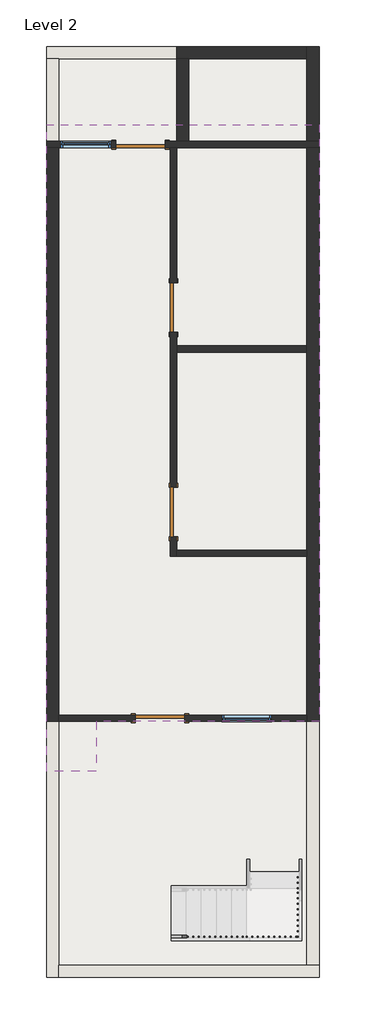
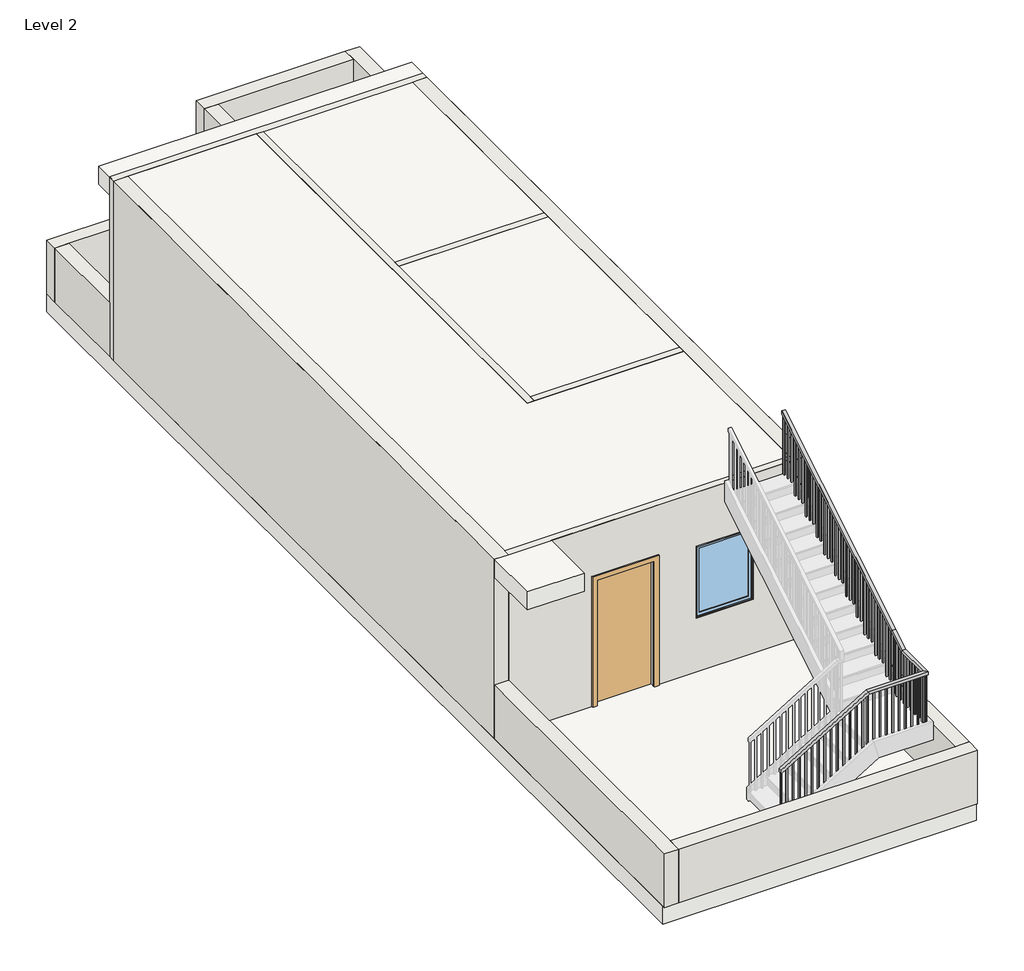
# One storey, part 1 of 2: 15 walls, 4 doors, 2 slabs, 2 windows, 1 railing.
"""IFC4 building model written with IfcOpenShell, lengths in millimetres."""

from ifc_helpers import new_model, si_unit, frame, origin, place, context, project, spatial, polyline, outline, extrude, faceted_brep, transform, mapped, element, save
from components import door_e5f9f3c4, window_41a96561

model = new_model("IFC4")

# Units and contexts
model_context = context("Model", 3, world=origin())
ifc_project = project(units=[si_unit("LENGTHUNIT", "METRE", prefix="MILLI")], contexts=[model_context])

# Site, building, storey
site = spatial("IfcSite", under=ifc_project)
building = spatial("IfcBuilding", under=site)
storey = spatial("IfcBuildingStorey", under=building, Name="Level 2", Elevation=3048.0)

# Doors
placement = place(None, origin())
door_shape = door_e5f9f3c4(model_context)
element("IfcDoor", 1, ObjectType="Single-Flush : 36\" x 84\"", at=placement, inside=storey, context=model_context, shape_type="MappedRepresentation", body=[
    mapped(door_shape, transform((-3555.9766939, -8657.0597562, 3048.0), x_axis=(1.0, 0.0, 0.0), y_axis=(0.0, 1.0, 0.0), z_axis=(0.0, 0.0, 1.0))),
])
element("IfcDoor", 2, ObjectType="Single-Flush : 36\" x 84\"", at=placement, inside=storey, context=model_context, shape_type="MappedRepresentation", body=[
    mapped(door_shape, transform((-3917.9266939, 1934.7402438, 3048.0), x_axis=(-1.0, 0.0, 0.0), y_axis=(0.0, -1.0, 0.0), z_axis=(0.0, 0.0, 1.0))),
])
element("IfcDoor", 3, ObjectType="Single-Flush : 36\" x 84\"", at=placement, inside=storey, context=model_context, shape_type="MappedRepresentation", body=[
    mapped(door_shape, transform((-3308.3266939, -1075.1597562, 3048.0), x_axis=(0.0, 1.0, 0.0), y_axis=(-1.0, 0.0, 0.0), z_axis=(0.0, 0.0, 1.0))),
])
element("IfcDoor", 4, ObjectType="Single-Flush : 36\" x 84\"", at=placement, inside=storey, context=model_context, shape_type="MappedRepresentation", body=[
    mapped(door_shape, transform((-3308.3266939, -4847.0597562, 3048.0), x_axis=(0.0, 1.0, 0.0), y_axis=(-1.0, 0.0, 0.0), z_axis=(0.0, 0.0, 1.0))),
])

# Railing
element("IfcRailing", 5, ObjectType="Handrail - Rectangular", at=placement, inside=storey, context=model_context, shape_type="SolidModel", body=[
    faceted_brep([(-3351.0563134, -12658.659218, 4131.7333333), (-3351.0563134, -12658.659218, 4072.3318731), (-3351.0563134, -12709.459218, 4072.3318731), (-3351.0563134, -12709.459218, 4131.7333333), (-1954.0563134, -12658.659218, 4978.4), (-1939.863904, -12658.659218, 4927.6), (-1939.863904, -12709.459218, 4927.6), (-1954.0563134, -12709.459218, 4978.4), (-1039.6563134, -12658.659218, 4978.4), (-1039.6563134, -12658.659218, 4927.6), (-988.8563134, -12709.459218, 4927.6), (-988.8563134, -12709.459218, 4978.4), (-1039.6563134, -12074.459218, 4978.4), (-1039.6563134, -12060.2668086, 4927.6), (-988.8563134, -12060.2668086, 4927.6), (-988.8563134, -12074.459218, 4978.4), (-1039.6563134, -11795.059218, 5147.7333333), (-1039.6563134, -11768.7294908, 5104.2892835), (-988.8563134, -11768.7294908, 5104.2892835), (-988.8563134, -11795.059218, 5147.7333333), (-1039.6563134, -8721.659218, 7010.4), (-988.8563134, -8721.659218, 7010.4), (-988.8563134, -8721.659218, 6950.9985397), (-1039.6563134, -8721.659218, 6950.9985397)], [[[0, 1, 2, 3]], [[1, 0, 4, 5]], [[2, 1, 5, 6]], [[3, 2, 6, 7]], [[0, 3, 7, 4]], [[5, 4, 8, 9]], [[6, 5, 9, 10]], [[7, 6, 10, 11]], [[4, 7, 11, 8]], [[9, 8, 12, 13]], [[10, 9, 13, 14]], [[11, 10, 14, 15]], [[8, 11, 15, 12]], [[13, 12, 16, 17]], [[14, 13, 17, 18]], [[15, 14, 18, 19]], [[12, 15, 19, 16]], [[20, 21, 22, 23]], [[17, 16, 20, 23]], [[18, 17, 23, 22]], [[19, 18, 22, 21]], [[16, 19, 21, 20]]]),
    extrude(outline(polyline([(-8756.584218, 6929.8318731), (-8737.534218, 6941.3773276), (-8737.534218, 5926.6666667), (-8756.584218, 5926.6666667), (-8756.584218, 6929.8318731)])), frame((-1023.7813134, 0.0, 0.0), z_axis=(1.0, 0.0, 0.0), x_axis=(0.0, 1.0, 0.0)), (0.0, 0.0, 1.0), 19.05),
    extrude(outline(polyline([(-8858.184218, 6868.2561155), (-8839.134218, 6879.80157), (-8839.134218, 5926.6666667), (-8858.184218, 5926.6666667), (-8858.184218, 6868.2561155)])), frame((-1023.7813134, 0.0, 0.0), z_axis=(1.0, 0.0, 0.0), x_axis=(0.0, 1.0, 0.0)), (0.0, 0.0, 1.0), 19.05),
    extrude(outline(polyline([(-8959.784218, 6806.6803579), (-8940.734218, 6818.2258125), (-8940.734218, 5926.6666667), (-8959.784218, 5926.6666667), (-8959.784218, 6806.6803579)])), frame((-1023.7813134, 0.0, 0.0), z_axis=(1.0, 0.0, 0.0), x_axis=(0.0, 1.0, 0.0)), (0.0, 0.0, 1.0), 19.05),
    extrude(outline(polyline([(-9061.384218, 6745.1046004), (-9042.334218, 6756.6500549), (-9042.334218, 5757.3333333), (-9061.384218, 5757.3333333), (-9061.384218, 6745.1046004)])), frame((-1023.7813134, 0.0, 0.0), z_axis=(1.0, 0.0, 0.0), x_axis=(0.0, 1.0, 0.0)), (0.0, 0.0, 1.0), 19.05),
    extrude(outline(polyline([(-9162.984218, 6683.5288428), (-9143.934218, 6695.0742973), (-9143.934218, 5757.3333333), (-9162.984218, 5757.3333333), (-9162.984218, 6683.5288428)])), frame((-1023.7813134, 0.0, 0.0), z_axis=(1.0, 0.0, 0.0), x_axis=(0.0, 1.0, 0.0)), (0.0, 0.0, 1.0), 19.05),
    extrude(outline(polyline([(-9264.584218, 6621.9530852), (-9245.534218, 6633.4985397), (-9245.534218, 5757.3333333), (-9264.584218, 5757.3333333), (-9264.584218, 6621.9530852)])), frame((-1023.7813134, 0.0, 0.0), z_axis=(1.0, 0.0, 0.0), x_axis=(0.0, 1.0, 0.0)), (0.0, 0.0, 1.0), 19.05),
    extrude(outline(polyline([(-9366.184218, 6560.3773276), (-9347.134218, 6571.9227822), (-9347.134218, 5588.0), (-9366.184218, 5588.0), (-9366.184218, 6560.3773276)])), frame((-1023.7813134, 0.0, 0.0), z_axis=(1.0, 0.0, 0.0), x_axis=(0.0, 1.0, 0.0)), (0.0, 0.0, 1.0), 19.05),
    extrude(outline(polyline([(-9467.784218, 6498.80157), (-9448.734218, 6510.3470246), (-9448.734218, 5588.0), (-9467.784218, 5588.0), (-9467.784218, 6498.80157)])), frame((-1023.7813134, 0.0, 0.0), z_axis=(1.0, 0.0, 0.0), x_axis=(0.0, 1.0, 0.0)), (0.0, 0.0, 1.0), 19.05),
    extrude(outline(polyline([(-9569.384218, 6437.2258125), (-9550.334218, 6448.771267), (-9550.334218, 5588.0), (-9569.384218, 5588.0), (-9569.384218, 6437.2258125)])), frame((-1023.7813134, 0.0, 0.0), z_axis=(1.0, 0.0, 0.0), x_axis=(0.0, 1.0, 0.0)), (0.0, 0.0, 1.0), 19.05),
    extrude(outline(polyline([(-9670.984218, 6375.6500549), (-9651.934218, 6387.1955094), (-9651.934218, 5418.6666667), (-9670.984218, 5418.6666667), (-9670.984218, 6375.6500549)])), frame((-1023.7813134, 0.0, 0.0), z_axis=(1.0, 0.0, 0.0), x_axis=(0.0, 1.0, 0.0)), (0.0, 0.0, 1.0), 19.05),
    extrude(outline(polyline([(-9772.584218, 6314.0742973), (-9753.534218, 6325.6197519), (-9753.534218, 5418.6666667), (-9772.584218, 5418.6666667), (-9772.584218, 6314.0742973)])), frame((-1023.7813134, 0.0, 0.0), z_axis=(1.0, 0.0, 0.0), x_axis=(0.0, 1.0, 0.0)), (0.0, 0.0, 1.0), 19.05),
    extrude(outline(polyline([(-9874.184218, 6252.4985397), (-9855.134218, 6264.0439943), (-9855.134218, 5249.3333333), (-9874.184218, 5249.3333333), (-9874.184218, 6252.4985397)])), frame((-1023.7813134, 0.0, 0.0), z_axis=(1.0, 0.0, 0.0), x_axis=(0.0, 1.0, 0.0)), (0.0, 0.0, 1.0), 19.05),
    extrude(outline(polyline([(-9975.784218, 6190.9227822), (-9956.734218, 6202.4682367), (-9956.734218, 5249.3333333), (-9975.784218, 5249.3333333), (-9975.784218, 6190.9227822)])), frame((-1023.7813134, 0.0, 0.0), z_axis=(1.0, 0.0, 0.0), x_axis=(0.0, 1.0, 0.0)), (0.0, 0.0, 1.0), 19.05),
    extrude(outline(polyline([(-10077.384218, 6129.3470246), (-10058.334218, 6140.8924791), (-10058.334218, 5249.3333333), (-10077.384218, 5249.3333333), (-10077.384218, 6129.3470246)])), frame((-1023.7813134, 0.0, 0.0), z_axis=(1.0, 0.0, 0.0), x_axis=(0.0, 1.0, 0.0)), (0.0, 0.0, 1.0), 19.05),
    extrude(outline(polyline([(-10178.984218, 6067.771267), (-10159.934218, 6079.3167216), (-10159.934218, 5080.0), (-10178.984218, 5080.0), (-10178.984218, 6067.771267)])), frame((-1023.7813134, 0.0, 0.0), z_axis=(1.0, 0.0, 0.0), x_axis=(0.0, 1.0, 0.0)), (0.0, 0.0, 1.0), 19.05),
    extrude(outline(polyline([(-10280.584218, 6006.1955094), (-10261.534218, 6017.740964), (-10261.534218, 5080.0), (-10280.584218, 5080.0), (-10280.584218, 6006.1955094)])), frame((-1023.7813134, 0.0, 0.0), z_axis=(1.0, 0.0, 0.0), x_axis=(0.0, 1.0, 0.0)), (0.0, 0.0, 1.0), 19.05),
    extrude(outline(polyline([(-10382.184218, 5944.6197519), (-10363.134218, 5956.1652064), (-10363.134218, 5080.0), (-10382.184218, 5080.0), (-10382.184218, 5944.6197519)])), frame((-1023.7813134, 0.0, 0.0), z_axis=(1.0, 0.0, 0.0), x_axis=(0.0, 1.0, 0.0)), (0.0, 0.0, 1.0), 19.05),
    extrude(outline(polyline([(-10483.784218, 5883.0439943), (-10464.734218, 5894.5894488), (-10464.734218, 4910.6666667), (-10483.784218, 4910.6666667), (-10483.784218, 5883.0439943)])), frame((-1023.7813134, 0.0, 0.0), z_axis=(1.0, 0.0, 0.0), x_axis=(0.0, 1.0, 0.0)), (0.0, 0.0, 1.0), 19.05),
    extrude(outline(polyline([(-10585.384218, 5821.4682367), (-10566.334218, 5833.0136913), (-10566.334218, 4910.6666667), (-10585.384218, 4910.6666667), (-10585.384218, 5821.4682367)])), frame((-1023.7813134, 0.0, 0.0), z_axis=(1.0, 0.0, 0.0), x_axis=(0.0, 1.0, 0.0)), (0.0, 0.0, 1.0), 19.05),
    extrude(outline(polyline([(-10686.984218, 5759.8924791), (-10667.934218, 5771.4379337), (-10667.934218, 4910.6666667), (-10686.984218, 4910.6666667), (-10686.984218, 5759.8924791)])), frame((-1023.7813134, 0.0, 0.0), z_axis=(1.0, 0.0, 0.0), x_axis=(0.0, 1.0, 0.0)), (0.0, 0.0, 1.0), 19.05),
    extrude(outline(polyline([(-10788.584218, 5698.3167216), (-10769.534218, 5709.8621761), (-10769.534218, 4741.3333333), (-10788.584218, 4741.3333333), (-10788.584218, 5698.3167216)])), frame((-1023.7813134, 0.0, 0.0), z_axis=(1.0, 0.0, 0.0), x_axis=(0.0, 1.0, 0.0)), (0.0, 0.0, 1.0), 19.05),
    extrude(outline(polyline([(-10890.184218, 5636.740964), (-10871.134218, 5648.2864185), (-10871.134218, 4741.3333333), (-10890.184218, 4741.3333333), (-10890.184218, 5636.740964)])), frame((-1023.7813134, 0.0, 0.0), z_axis=(1.0, 0.0, 0.0), x_axis=(0.0, 1.0, 0.0)), (0.0, 0.0, 1.0), 19.05),
    extrude(outline(polyline([(-10991.784218, 5575.1652064), (-10972.734218, 5586.710661), (-10972.734218, 4572.0), (-10991.784218, 4572.0), (-10991.784218, 5575.1652064)])), frame((-1023.7813134, 0.0, 0.0), z_axis=(1.0, 0.0, 0.0), x_axis=(0.0, 1.0, 0.0)), (0.0, 0.0, 1.0), 19.05),
    extrude(outline(polyline([(-11093.384218, 5513.5894488), (-11074.334218, 5525.1349034), (-11074.334218, 4572.0), (-11093.384218, 4572.0), (-11093.384218, 5513.5894488)])), frame((-1023.7813134, 0.0, 0.0), z_axis=(1.0, 0.0, 0.0), x_axis=(0.0, 1.0, 0.0)), (0.0, 0.0, 1.0), 19.05),
    extrude(outline(polyline([(-11194.984218, 5452.0136913), (-11175.934218, 5463.5591458), (-11175.934218, 4572.0), (-11194.984218, 4572.0), (-11194.984218, 5452.0136913)])), frame((-1023.7813134, 0.0, 0.0), z_axis=(1.0, 0.0, 0.0), x_axis=(0.0, 1.0, 0.0)), (0.0, 0.0, 1.0), 19.05),
    extrude(outline(polyline([(-11296.584218, 5390.4379337), (-11277.534218, 5401.9833882), (-11277.534218, 4402.6666667), (-11296.584218, 4402.6666667), (-11296.584218, 5390.4379337)])), frame((-1023.7813134, 0.0, 0.0), z_axis=(1.0, 0.0, 0.0), x_axis=(0.0, 1.0, 0.0)), (0.0, 0.0, 1.0), 19.05),
    extrude(outline(polyline([(-11398.184218, 5328.8621761), (-11379.134218, 5340.4076307), (-11379.134218, 4402.6666667), (-11398.184218, 4402.6666667), (-11398.184218, 5328.8621761)])), frame((-1023.7813134, 0.0, 0.0), z_axis=(1.0, 0.0, 0.0), x_axis=(0.0, 1.0, 0.0)), (0.0, 0.0, 1.0), 19.05),
    extrude(outline(polyline([(-11499.784218, 5267.2864185), (-11480.734218, 5278.8318731), (-11480.734218, 4402.6666667), (-11499.784218, 4402.6666667), (-11499.784218, 5267.2864185)])), frame((-1023.7813134, 0.0, 0.0), z_axis=(1.0, 0.0, 0.0), x_axis=(0.0, 1.0, 0.0)), (0.0, 0.0, 1.0), 19.05),
    extrude(outline(polyline([(-11601.384218, 5205.710661), (-11582.334218, 5217.2561155), (-11582.334218, 4233.3333333), (-11601.384218, 4233.3333333), (-11601.384218, 5205.710661)])), frame((-1023.7813134, 0.0, 0.0), z_axis=(1.0, 0.0, 0.0), x_axis=(0.0, 1.0, 0.0)), (0.0, 0.0, 1.0), 19.05),
    extrude(outline(polyline([(-11702.984218, 5144.1349034), (-11683.934218, 5155.6803579), (-11683.934218, 4233.3333333), (-11702.984218, 4233.3333333), (-11702.984218, 5144.1349034)])), frame((-1023.7813134, 0.0, 0.0), z_axis=(1.0, 0.0, 0.0), x_axis=(0.0, 1.0, 0.0)), (0.0, 0.0, 1.0), 19.05),
    extrude(outline(polyline([(-11880.784218, 5036.3773276), (-11861.734218, 5047.9227822), (-11861.734218, 4064.0), (-11880.784218, 4064.0), (-11880.784218, 5036.3773276)])), frame((-1023.7813134, 0.0, 0.0), z_axis=(1.0, 0.0, 0.0), x_axis=(0.0, 1.0, 0.0)), (0.0, 0.0, 1.0), 19.05),
    extrude(outline(polyline([(-11982.384218, 4974.80157), (-11963.334218, 4986.3470246), (-11963.334218, 4064.0), (-11982.384218, 4064.0), (-11982.384218, 4974.80157)])), frame((-1023.7813134, 0.0, 0.0), z_axis=(1.0, 0.0, 0.0), x_axis=(0.0, 1.0, 0.0)), (0.0, 0.0, 1.0), 19.05),
    extrude(outline(polyline([(-1004.7313134, -12083.984218), (-1023.7813134, -12083.984218), (-1023.7813134, -12064.934218), (-1004.7313134, -12064.934218), (-1004.7313134, -12083.984218)])), frame((0.0, 0.0, 4064.0), z_axis=(0.0, 0.0, 1.0), x_axis=(1.0, 0.0, 0.0)), (0.0, 0.0, 1.0), 863.6),
    extrude(outline(polyline([(-1004.7313134, -12185.584218), (-1023.7813134, -12185.584218), (-1023.7813134, -12166.534218), (-1004.7313134, -12166.534218), (-1004.7313134, -12185.584218)])), frame((0.0, 0.0, 4064.0), z_axis=(0.0, 0.0, 1.0), x_axis=(1.0, 0.0, 0.0)), (0.0, 0.0, 1.0), 863.6),
    extrude(outline(polyline([(-1004.7313134, -12287.184218), (-1023.7813134, -12287.184218), (-1023.7813134, -12268.134218), (-1004.7313134, -12268.134218), (-1004.7313134, -12287.184218)])), frame((0.0, 0.0, 4064.0), z_axis=(0.0, 0.0, 1.0), x_axis=(1.0, 0.0, 0.0)), (0.0, 0.0, 1.0), 863.6),
    extrude(outline(polyline([(-1004.7313134, -12388.784218), (-1023.7813134, -12388.784218), (-1023.7813134, -12369.734218), (-1004.7313134, -12369.734218), (-1004.7313134, -12388.784218)])), frame((0.0, 0.0, 4064.0), z_axis=(0.0, 0.0, 1.0), x_axis=(1.0, 0.0, 0.0)), (0.0, 0.0, 1.0), 863.6),
    extrude(outline(polyline([(-1004.7313134, -12490.384218), (-1023.7813134, -12490.384218), (-1023.7813134, -12471.334218), (-1004.7313134, -12471.334218), (-1004.7313134, -12490.384218)])), frame((0.0, 0.0, 4064.0), z_axis=(0.0, 0.0, 1.0), x_axis=(1.0, 0.0, 0.0)), (0.0, 0.0, 1.0), 863.6),
    extrude(outline(polyline([(-1004.7313134, -12591.984218), (-1023.7813134, -12591.984218), (-1023.7813134, -12572.934218), (-1004.7313134, -12572.934218), (-1004.7313134, -12591.984218)])), frame((0.0, 0.0, 4064.0), z_axis=(0.0, 0.0, 1.0), x_axis=(1.0, 0.0, 0.0)), (0.0, 0.0, 1.0), 863.6),
    extrude(outline(polyline([(-1049.1813134, -12693.584218), (-1049.1813134, -12674.534218), (-1030.1313134, -12674.534218), (-1030.1313134, -12693.584218), (-1049.1813134, -12693.584218)])), frame((0.0, 0.0, 4064.0), z_axis=(0.0, 0.0, 1.0), x_axis=(1.0, 0.0, 0.0)), (0.0, 0.0, 1.0), 863.6),
    extrude(outline(polyline([(-1150.7813134, -12693.584218), (-1150.7813134, -12674.534218), (-1131.7313134, -12674.534218), (-1131.7313134, -12693.584218), (-1150.7813134, -12693.584218)])), frame((0.0, 0.0, 4064.0), z_axis=(0.0, 0.0, 1.0), x_axis=(1.0, 0.0, 0.0)), (0.0, 0.0, 1.0), 863.6),
    extrude(outline(polyline([(-1252.3813134, -12693.584218), (-1252.3813134, -12674.534218), (-1233.3313134, -12674.534218), (-1233.3313134, -12693.584218), (-1252.3813134, -12693.584218)])), frame((0.0, 0.0, 4064.0), z_axis=(0.0, 0.0, 1.0), x_axis=(1.0, 0.0, 0.0)), (0.0, 0.0, 1.0), 863.6),
    extrude(outline(polyline([(-1353.9813134, -12693.584218), (-1353.9813134, -12674.534218), (-1334.9313134, -12674.534218), (-1334.9313134, -12693.584218), (-1353.9813134, -12693.584218)])), frame((0.0, 0.0, 4064.0), z_axis=(0.0, 0.0, 1.0), x_axis=(1.0, 0.0, 0.0)), (0.0, 0.0, 1.0), 863.6),
    extrude(outline(polyline([(-1455.5813134, -12693.584218), (-1455.5813134, -12674.534218), (-1436.5313134, -12674.534218), (-1436.5313134, -12693.584218), (-1455.5813134, -12693.584218)])), frame((0.0, 0.0, 4064.0), z_axis=(0.0, 0.0, 1.0), x_axis=(1.0, 0.0, 0.0)), (0.0, 0.0, 1.0), 863.6),
    extrude(outline(polyline([(-1557.1813134, -12693.584218), (-1557.1813134, -12674.534218), (-1538.1313134, -12674.534218), (-1538.1313134, -12693.584218), (-1557.1813134, -12693.584218)])), frame((0.0, 0.0, 4064.0), z_axis=(0.0, 0.0, 1.0), x_axis=(1.0, 0.0, 0.0)), (0.0, 0.0, 1.0), 863.6),
    extrude(outline(polyline([(-1658.7813134, -12693.584218), (-1658.7813134, -12674.534218), (-1639.7313134, -12674.534218), (-1639.7313134, -12693.584218), (-1658.7813134, -12693.584218)])), frame((0.0, 0.0, 4064.0), z_axis=(0.0, 0.0, 1.0), x_axis=(1.0, 0.0, 0.0)), (0.0, 0.0, 1.0), 863.6),
    extrude(outline(polyline([(-1760.3813134, -12693.584218), (-1760.3813134, -12674.534218), (-1741.3313134, -12674.534218), (-1741.3313134, -12693.584218), (-1760.3813134, -12693.584218)])), frame((0.0, 0.0, 4064.0), z_axis=(0.0, 0.0, 1.0), x_axis=(1.0, 0.0, 0.0)), (0.0, 0.0, 1.0), 863.6),
    extrude(outline(polyline([(-1861.9813134, -12693.584218), (-1861.9813134, -12674.534218), (-1842.9313134, -12674.534218), (-1842.9313134, -12693.584218), (-1861.9813134, -12693.584218)])), frame((0.0, 0.0, 4064.0), z_axis=(0.0, 0.0, 1.0), x_axis=(1.0, 0.0, 0.0)), (0.0, 0.0, 1.0), 863.6),
    extrude(outline(polyline([(4878.5894488, -2020.7313134), (4867.0439943, -2039.7813134), (3894.6666667, -2039.7813134), (3894.6666667, -2020.7313134), (4878.5894488, -2020.7313134)])), frame((0.0, -12693.584218, 0.0), z_axis=(0.0, 1.0, 0.0), x_axis=(0.0, 0.0, 1.0)), (0.0, 0.0, 1.0), 19.05),
    extrude(outline(polyline([(4817.0136913, -2122.3313134), (4805.4682367, -2141.3813134), (3894.6666667, -2141.3813134), (3894.6666667, -2122.3313134), (4817.0136913, -2122.3313134)])), frame((0.0, -12693.584218, 0.0), z_axis=(0.0, 1.0, 0.0), x_axis=(0.0, 0.0, 1.0)), (0.0, 0.0, 1.0), 19.05),
    extrude(outline(polyline([(4755.4379337, -2223.9313134), (4743.8924791, -2242.9813134), (3894.6666667, -2242.9813134), (3894.6666667, -2223.9313134), (4755.4379337, -2223.9313134)])), frame((0.0, -12693.584218, 0.0), z_axis=(0.0, 1.0, 0.0), x_axis=(0.0, 0.0, 1.0)), (0.0, 0.0, 1.0), 19.05),
    extrude(outline(polyline([(4693.8621761, -2325.5313134), (4682.3167216, -2344.5813134), (3725.3333333, -2344.5813134), (3725.3333333, -2325.5313134), (4693.8621761, -2325.5313134)])), frame((0.0, -12693.584218, 0.0), z_axis=(0.0, 1.0, 0.0), x_axis=(0.0, 0.0, 1.0)), (0.0, 0.0, 1.0), 19.05),
    extrude(outline(polyline([(4632.2864185, -2427.1313134), (4620.740964, -2446.1813134), (3725.3333333, -2446.1813134), (3725.3333333, -2427.1313134), (4632.2864185, -2427.1313134)])), frame((0.0, -12693.584218, 0.0), z_axis=(0.0, 1.0, 0.0), x_axis=(0.0, 0.0, 1.0)), (0.0, 0.0, 1.0), 19.05),
    extrude(outline(polyline([(4570.710661, -2528.7313134), (4559.1652064, -2547.7813134), (3556.0, -2547.7813134), (3556.0, -2528.7313134), (4570.710661, -2528.7313134)])), frame((0.0, -12693.584218, 0.0), z_axis=(0.0, 1.0, 0.0), x_axis=(0.0, 0.0, 1.0)), (0.0, 0.0, 1.0), 19.05),
    extrude(outline(polyline([(4509.1349034, -2630.3313134), (4497.5894488, -2649.3813134), (3556.0, -2649.3813134), (3556.0, -2630.3313134), (4509.1349034, -2630.3313134)])), frame((0.0, -12693.584218, 0.0), z_axis=(0.0, 1.0, 0.0), x_axis=(0.0, 0.0, 1.0)), (0.0, 0.0, 1.0), 19.05),
    extrude(outline(polyline([(4447.5591458, -2731.9313134), (4436.0136913, -2750.9813134), (3556.0, -2750.9813134), (3556.0, -2731.9313134), (4447.5591458, -2731.9313134)])), frame((0.0, -12693.584218, 0.0), z_axis=(0.0, 1.0, 0.0), x_axis=(0.0, 0.0, 1.0)), (0.0, 0.0, 1.0), 19.05),
    extrude(outline(polyline([(4385.9833882, -2833.5313134), (4374.4379337, -2852.5813134), (3386.6666667, -2852.5813134), (3386.6666667, -2833.5313134), (4385.9833882, -2833.5313134)])), frame((0.0, -12693.584218, 0.0), z_axis=(0.0, 1.0, 0.0), x_axis=(0.0, 0.0, 1.0)), (0.0, 0.0, 1.0), 19.05),
    extrude(outline(polyline([(4324.4076307, -2935.1313134), (4312.8621761, -2954.1813134), (3386.6666667, -2954.1813134), (3386.6666667, -2935.1313134), (4324.4076307, -2935.1313134)])), frame((0.0, -12693.584218, 0.0), z_axis=(0.0, 1.0, 0.0), x_axis=(0.0, 0.0, 1.0)), (0.0, 0.0, 1.0), 19.05),
    extrude(outline(polyline([(4262.8318731, -3036.7313134), (4251.2864185, -3055.7813134), (3386.6666667, -3055.7813134), (3386.6666667, -3036.7313134), (4262.8318731, -3036.7313134)])), frame((0.0, -12693.584218, 0.0), z_axis=(0.0, 1.0, 0.0), x_axis=(0.0, 0.0, 1.0)), (0.0, 0.0, 1.0), 19.05),
    extrude(outline(polyline([(4201.2561155, -3138.3313134), (4189.710661, -3157.3813134), (3217.3333333, -3157.3813134), (3217.3333333, -3138.3313134), (4201.2561155, -3138.3313134)])), frame((0.0, -12693.584218, 0.0), z_axis=(0.0, 1.0, 0.0), x_axis=(0.0, 0.0, 1.0)), (0.0, 0.0, 1.0), 19.05),
    extrude(outline(polyline([(4139.6803579, -3239.9313134), (4128.1349034, -3258.9813134), (3217.3333333, -3258.9813134), (3217.3333333, -3239.9313134), (4139.6803579, -3239.9313134)])), frame((0.0, -12693.584218, 0.0), z_axis=(0.0, 1.0, 0.0), x_axis=(0.0, 0.0, 1.0)), (0.0, 0.0, 1.0), 19.05),
    extrude(outline(polyline([(-11804.584218, 5082.5591458), (-11785.534218, 5094.1046004), (-11785.534218, 4064.0), (-11804.584218, 4064.0), (-11804.584218, 5082.5591458)])), frame((-1023.7813134, 0.0, 0.0), z_axis=(1.0, 0.0, 0.0), x_axis=(0.0, 1.0, 0.0)), (0.0, 0.0, 1.0), 19.05),
    extrude(outline(polyline([(-1023.7813134, -12693.584218), (-1023.7813134, -12674.534218), (-1004.7313134, -12674.534218), (-1004.7313134, -12693.584218), (-1023.7813134, -12693.584218)])), frame((0.0, 0.0, 4064.0), z_axis=(0.0, 0.0, 1.0), x_axis=(1.0, 0.0, 0.0)), (0.0, 0.0, 1.0), 863.6),
    extrude(outline(polyline([(4924.771267, -1944.5313134), (4913.2258125, -1963.5813134), (4064.0, -1963.5813134), (4064.0, -1944.5313134), (4924.771267, -1944.5313134)])), frame((0.0, -12693.584218, 0.0), z_axis=(0.0, 1.0, 0.0), x_axis=(0.0, 0.0, 1.0)), (0.0, 0.0, 1.0), 19.05),
    extrude(outline(polyline([(-8740.709218, 6939.4530852), (-8721.659218, 6950.9985397), (-8721.659218, 5926.6666667), (-8740.709218, 5926.6666667), (-8740.709218, 6939.4530852)])), frame((-1023.7813134, 0.0, 0.0), z_axis=(1.0, 0.0, 0.0), x_axis=(0.0, 1.0, 0.0)), (0.0, 0.0, 1.0), 19.05),
    extrude(outline(polyline([(4083.8773276, -3332.0063134), (4072.3318731, -3351.0563134), (3217.3333333, -3351.0563134), (3217.3333333, -3332.0063134), (4083.8773276, -3332.0063134)])), frame((0.0, -12693.584218, 0.0), z_axis=(0.0, 1.0, 0.0), x_axis=(0.0, 0.0, 1.0)), (0.0, 0.0, 1.0), 19.05),
])

# Slabs
element("IfcSlab", 6, ObjectType="slab 6\"", at=placement, inside=storey, context=model_context, shape_type="SweptSolid", body=[
    extrude(outline(polyline([(-622.2766939, 3744.4902438), (-622.2766939, -13400.5097562), (-5651.4766939, -13400.5097562), (-5651.4766939, 3744.4902438), (-622.2766939, 3744.4902438)])), frame((0.0, 0.0, 2743.2), z_axis=(0.0, 0.0, 1.0), x_axis=(1.0, 0.0, 0.0)), (0.0, 0.0, 1.0), 304.8),
])
element("IfcSlab", 7, ObjectType="slab 6\"", at=placement, inside=storey, context=model_context, shape_type="SweptSolid", body=[
    extrude(outline(polyline([(-622.2766939, 2296.6902438), (-622.2766939, -8714.2097562), (-4737.0766939, -8714.2097562), (-4737.0766939, -9628.6097562), (-5651.4766939, -9628.6097562), (-5651.4766939, -8714.2097562), (-5651.4766939, 2296.6902438), (-622.2766939, 2296.6902438)])), frame((0.0, 0.0, 5791.2), z_axis=(0.0, 0.0, 1.0), x_axis=(1.0, 0.0, 0.0)), (0.0, 0.0, 1.0), 304.8),
])

# Walls
element("IfcWall", 8, ObjectType="wall 4.5\"", at=placement, inside=storey, context=model_context, shape_type="Brep", body=[
    faceted_brep([(-5651.4766939, 1877.5902438, 3048.0), (-5422.8766939, 1877.5902438, 3048.0), (-4375.1266939, 1877.5902438, 3048.0), (-4375.1266939, 1877.5902438, 5181.6), (-3460.7266939, 1877.5902438, 5181.6), (-3460.7266939, 1877.5902438, 3048.0), (-3365.4766939, 1877.5902438, 3048.0), (-3251.1766939, 1877.5902438, 3048.0), (-850.8766939, 1877.5902438, 3048.0), (-622.2766939, 1877.5902438, 3048.0), (-622.2766939, 1877.5902438, 6096.0), (-850.8766939, 1877.5902438, 6096.0), (-3251.1766939, 1877.5902438, 6096.0), (-3365.4766939, 1877.5902438, 6096.0), (-5422.8766939, 1877.5902438, 6096.0), (-5651.4766939, 1877.5902438, 6096.0), (-4470.3766939, 1877.5902438, 5181.6), (-4470.3766939, 1877.5902438, 3962.4), (-5384.7766939, 1877.5902438, 3962.4), (-5384.7766939, 1877.5902438, 5181.6), (-4375.1266939, 1991.8902438, 5181.6), (-4375.1266939, 1991.8902438, 3048.0), (-5422.8766939, 1991.8902438, 3048.0), (-5651.4766939, 1991.8902438, 3048.0), (-5651.4766939, 1991.8902438, 3962.4), (-5651.4766939, 1991.8902438, 6096.0), (-622.2766939, 1991.8902438, 6096.0), (-622.2766939, 1991.8902438, 5486.4), (-622.2766939, 1991.8902438, 3048.0), (-850.8766939, 1991.8902438, 3048.0), (-3022.5766939, 1991.8902438, 3048.0), (-3251.1766939, 1991.8902438, 3048.0), (-3460.7266939, 1991.8902438, 3048.0), (-3460.7266939, 1991.8902438, 5181.6), (-4470.3766939, 1991.8902438, 5181.6), (-5384.7766939, 1991.8902438, 5181.6), (-5384.7766939, 1991.8902438, 3962.4), (-4470.3766939, 1991.8902438, 3962.4)], [[[0, 1, 2, 3, 4, 5, 6, 7, 8, 9, 10, 11, 12, 13, 14, 15], [16, 17, 18, 19]], [[20, 21, 22, 23, 24, 25, 26, 27, 28, 29, 30, 31, 32, 33], [34, 35, 36, 37]], [[32, 31, 30, 29, 28, 9, 8, 7, 6, 5]], [[23, 22, 21, 2, 1, 0]], [[15, 14, 13, 12, 11, 10, 26, 25]], [[3, 2, 21, 20]], [[4, 3, 20, 33]], [[5, 4, 33, 32]], [[17, 16, 34, 37]], [[18, 17, 37, 36]], [[19, 18, 36, 35]], [[16, 19, 35, 34]], [[9, 28, 27, 26, 10]], [[15, 25, 24, 23, 0]]]),
])
element("IfcWall", 9, ObjectType="wall 4.5\"", at=placement, inside=storey, context=model_context, shape_type="Brep", body=[
    faceted_brep([(-3365.4766939, -1532.3597562, 3048.0), (-3365.4766939, -4389.8597562, 3048.0), (-3365.4766939, -4389.8597562, 5181.6), (-3365.4766939, -5304.2597562, 5181.6), (-3365.4766939, -5304.2597562, 3048.0), (-3365.4766939, -5666.2097562, 3048.0), (-3365.4766939, -5666.2097562, 6096.0), (-3365.4766939, 1877.5902438, 6096.0), (-3365.4766939, 1877.5902438, 3048.0), (-3365.4766939, -617.9597562, 3048.0), (-3365.4766939, -617.9597562, 5181.6), (-3365.4766939, -1532.3597562, 5181.6), (-3251.1766939, -4389.8597562, 5181.6), (-3251.1766939, -4389.8597562, 3048.0), (-3251.1766939, -1894.3097562, 3048.0), (-3251.1766939, -1780.0097562, 3048.0), (-3251.1766939, -1532.3597562, 3048.0), (-3251.1766939, -1532.3597562, 5181.6), (-3251.1766939, -617.9597562, 5181.6), (-3251.1766939, -617.9597562, 3048.0), (-3251.1766939, 1877.5902438, 3048.0), (-3251.1766939, 1877.5902438, 6096.0), (-3251.1766939, -1780.0097562, 6096.0), (-3251.1766939, -1894.3097562, 6096.0), (-3251.1766939, -5551.9097562, 6096.0), (-3251.1766939, -5666.2097562, 6096.0), (-3251.1766939, -5666.2097562, 3048.0), (-3251.1766939, -5551.9097562, 3048.0), (-3251.1766939, -5304.2597562, 3048.0), (-3251.1766939, -5304.2597562, 5181.6)], [[[0, 1, 2, 3, 4, 5, 6, 7, 8, 9, 10, 11]], [[12, 13, 14, 15, 16, 17, 18, 19, 20, 21, 22, 23, 24, 25, 26, 27, 28, 29]], [[20, 19, 9, 8]], [[28, 27, 26, 5, 4]], [[16, 15, 14, 13, 1, 0]], [[7, 6, 25, 24, 23, 22, 21]], [[8, 7, 21, 20]], [[6, 5, 26, 25]], [[10, 9, 19, 18]], [[11, 10, 18, 17]], [[0, 11, 17, 16]], [[2, 1, 13, 12]], [[3, 2, 12, 29]], [[4, 3, 29, 28]]]),
])
element("IfcWall", 10, ObjectType="wall 4.5\"", at=placement, inside=storey, context=model_context, shape_type="SweptSolid", body=[
    extrude(outline(polyline([(-3251.1766939, -5551.9097562), (-850.8766939, -5551.9097562), (-850.8766939, -5666.2097562), (-3251.1766939, -5666.2097562), (-3251.1766939, -5551.9097562)])), frame((0.0, 0.0, 3048.0), z_axis=(0.0, 0.0, 1.0), x_axis=(1.0, 0.0, 0.0)), (0.0, 0.0, 1.0), 3048.0),
])
element("IfcWall", 11, ObjectType="wall 4.5\"", at=placement, inside=storey, context=model_context, shape_type="SweptSolid", body=[
    extrude(outline(polyline([(-3251.1766939, -1780.0097562), (-850.8766939, -1780.0097562), (-850.8766939, -1894.3097562), (-3251.1766939, -1894.3097562), (-3251.1766939, -1780.0097562)])), frame((0.0, 0.0, 3048.0), z_axis=(0.0, 0.0, 1.0), x_axis=(1.0, 0.0, 0.0)), (0.0, 0.0, 1.0), 3048.0),
])
element("IfcWall", 12, ObjectType="wall 4.5\"", at=placement, inside=storey, context=model_context, shape_type="SweptSolid", body=[
    extrude(outline(polyline([(5181.6, -3098.7766939), (3048.0, -3098.7766939), (3048.0, -850.8766939), (6096.0, -850.8766939), (6096.0, -5422.8766939), (3048.0, -5422.8766939), (3048.0, -4013.1766939), (5181.6, -4013.1766939), (5181.6, -3098.7766939)]), holes=[polyline([(5181.6, -2412.9766939), (5181.6, -1498.5766939), (3962.4, -1498.5766939), (3962.4, -2412.9766939), (5181.6, -2412.9766939)])]), frame((0.0, -8714.2097562, 0.0), z_axis=(0.0, 1.0, 0.0), x_axis=(0.0, 0.0, 1.0)), (0.0, 0.0, 1.0), 114.3),
])
element("IfcWall", 13, ObjectType="wall 9\"", at=placement, inside=storey, context=model_context, shape_type="Brep", body=[
    faceted_brep([(-850.8766939, 1877.5902438, 6096.0), (-850.8766939, 1877.5902438, 3048.0), (-850.8766939, -1780.0097562, 3048.0), (-850.8766939, -1894.3097562, 3048.0), (-850.8766939, -5551.9097562, 3048.0), (-850.8766939, -5666.2097562, 3048.0), (-850.8766939, -8599.9097562, 3048.0), (-850.8766939, -8714.2097562, 3048.0), (-850.8766939, -8714.2097562, 3962.4), (-850.8766939, -8714.2097562, 6096.0), (-850.8766939, -8599.9097562, 6096.0), (-850.8766939, -5666.2097562, 6096.0), (-850.8766939, -5551.9097562, 6096.0), (-850.8766939, -1894.3097562, 6096.0), (-850.8766939, -1780.0097562, 6096.0), (-622.2766939, 1877.5902438, 3048.0), (-622.2766939, 1877.5902438, 6096.0), (-622.2766939, -8714.2097562, 6096.0), (-622.2766939, -8714.2097562, 3962.4), (-622.2766939, -8714.2097562, 3048.0)], [[[0, 1, 2, 3, 4, 5, 6, 7, 8, 9, 10, 11, 12, 13, 14]], [[15, 16, 17, 18, 19]], [[7, 6, 5, 4, 3, 2, 1, 15, 19]], [[0, 14, 13, 12, 11, 10, 9, 17, 16]], [[0, 16, 15, 1]], [[7, 19, 18, 17, 9, 8]]]),
])
element("IfcWall", 14, ObjectType="wall 9\"", at=placement, inside=storey, context=model_context, shape_type="Brep", body=[
    faceted_brep([(-5422.8766939, -8714.2097562, 6096.0), (-5422.8766939, -8714.2097562, 3962.4), (-5422.8766939, -8714.2097562, 3048.0), (-5422.8766939, -8599.9097562, 3048.0), (-5422.8766939, 1877.5902438, 3048.0), (-5422.8766939, 1877.5902438, 6096.0), (-5422.8766939, -8599.9097562, 6096.0), (-5651.4766939, -8714.2097562, 3048.0), (-5651.4766939, -8714.2097562, 3962.4), (-5651.4766939, -8714.2097562, 6096.0), (-5651.4766939, 1877.5902438, 6096.0), (-5651.4766939, 1877.5902438, 3048.0)], [[[0, 1, 2, 3, 4, 5, 6]], [[7, 8, 9, 10, 11]], [[4, 3, 2, 7, 11]], [[0, 6, 5, 10, 9]], [[4, 11, 10, 5]], [[0, 9, 8, 7, 2, 1]]]),
])
element("IfcWall", 15, ObjectType="wall 9\"", at=placement, inside=storey, context=model_context, shape_type="Brep", body=[
    faceted_brep([(-622.2766939, 1991.8902438, 3048.0), (-622.2766939, 3744.4902438, 3048.0), (-622.2766939, 3744.4902438, 5486.4), (-622.2766939, 1991.8902438, 5486.4), (-850.8766939, 1991.8902438, 3048.0), (-850.8766939, 1991.8902438, 5486.4), (-850.8766939, 3515.8902438, 5486.4), (-850.8766939, 3744.4902438, 5486.4), (-850.8766939, 3744.4902438, 3048.0), (-850.8766939, 3515.8902438, 3048.0)], [[[0, 1, 2, 3]], [[4, 5, 6, 7, 8, 9]], [[1, 0, 4, 9, 8]], [[3, 2, 7, 6, 5]], [[0, 3, 5, 4]], [[2, 1, 8, 7]]]),
])
element("IfcWall", 16, ObjectType="wall 9\"", at=placement, inside=storey, context=model_context, shape_type="Brep", body=[
    faceted_brep([(-850.8766939, 3744.4902438, 3048.0), (-3251.1766939, 3744.4902438, 3048.0), (-3251.1766939, 3744.4902438, 3962.4), (-3251.1766939, 3744.4902438, 5486.4), (-850.8766939, 3744.4902438, 5486.4), (-850.8766939, 3515.8902438, 3048.0), (-850.8766939, 3515.8902438, 5486.4), (-3022.5766939, 3515.8902438, 5486.4), (-3251.1766939, 3515.8902438, 5486.4), (-3251.1766939, 3515.8902438, 3962.4), (-3251.1766939, 3515.8902438, 3048.0), (-3022.5766939, 3515.8902438, 3048.0)], [[[0, 1, 2, 3, 4]], [[5, 6, 7, 8, 9, 10, 11]], [[1, 0, 5, 11, 10]], [[4, 3, 8, 7, 6]], [[0, 4, 6, 5]], [[1, 10, 9, 8, 3, 2]]]),
])
element("IfcWall", 17, ObjectType="wall 9\"", at=placement, inside=storey, context=model_context, shape_type="SweptSolid", body=[
    extrude(outline(polyline([(-3251.1766939, 1991.8902438), (-3251.1766939, 3515.8902438), (-3022.5766939, 3515.8902438), (-3022.5766939, 1991.8902438), (-3251.1766939, 1991.8902438)])), frame((0.0, 0.0, 3048.0), z_axis=(0.0, 0.0, 1.0), x_axis=(1.0, 0.0, 0.0)), (0.0, 0.0, 1.0), 2438.4),
])
element("IfcWall", 18, ObjectType="wall 9\"", at=placement, inside=storey, context=model_context, shape_type="Brep", body=[
    faceted_brep([(-3251.1766939, 3744.4902438, 3048.0), (-5651.4766939, 3744.4902438, 3048.0), (-5651.4766939, 3744.4902438, 3962.4), (-3251.1766939, 3744.4902438, 3962.4), (-3251.1766939, 3515.8902438, 3048.0), (-3251.1766939, 3515.8902438, 3962.4), (-5422.8766939, 3515.8902438, 3962.4), (-5651.4766939, 3515.8902438, 3962.4), (-5651.4766939, 3515.8902438, 3048.0), (-5422.8766939, 3515.8902438, 3048.0)], [[[0, 1, 2, 3]], [[4, 5, 6, 7, 8, 9]], [[1, 0, 4, 9, 8]], [[3, 2, 7, 6, 5]], [[0, 3, 5, 4]], [[2, 1, 8, 7]]]),
])
element("IfcWall", 19, ObjectType="wall 9\"", at=placement, inside=storey, context=model_context, shape_type="SweptSolid", body=[
    extrude(outline(polyline([(-5651.4766939, 1991.8902438), (-5651.4766939, 3515.8902438), (-5422.8766939, 3515.8902438), (-5422.8766939, 1991.8902438), (-5651.4766939, 1991.8902438)])), frame((0.0, 0.0, 3048.0), z_axis=(0.0, 0.0, 1.0), x_axis=(1.0, 0.0, 0.0)), (0.0, 0.0, 1.0), 914.4),
])
element("IfcWall", 20, ObjectType="wall 9\"", at=placement, inside=storey, context=model_context, shape_type="Brep", body=[
    faceted_brep([(-5651.4766939, -8714.2097562, 3048.0), (-5651.4766939, -13438.6097562, 3048.0), (-5651.4766939, -13438.6097562, 3962.4), (-5651.4766939, -8714.2097562, 3962.4), (-5422.8766939, -8714.2097562, 3048.0), (-5422.8766939, -8714.2097562, 3962.4), (-5422.8766939, -13210.0097562, 3962.4), (-5422.8766939, -13438.6097562, 3962.4), (-5422.8766939, -13438.6097562, 3048.0), (-5422.8766939, -13210.0097562, 3048.0)], [[[0, 1, 2, 3]], [[4, 5, 6, 7, 8, 9]], [[1, 0, 4, 9, 8]], [[3, 2, 7, 6, 5]], [[0, 3, 5, 4]], [[2, 1, 8, 7]]]),
])
element("IfcWall", 21, ObjectType="wall 9\"", at=placement, inside=storey, context=model_context, shape_type="Brep", body=[
    faceted_brep([(-5422.8766939, -13438.6097562, 3048.0), (-622.2766939, -13438.6097562, 3048.0), (-622.2766939, -13438.6097562, 3962.4), (-5422.8766939, -13438.6097562, 3962.4), (-5422.8766939, -13210.0097562, 3048.0), (-5422.8766939, -13210.0097562, 3962.4), (-850.8766939, -13210.0097562, 3962.4), (-622.2766939, -13210.0097562, 3962.4), (-622.2766939, -13210.0097562, 3048.0), (-850.8766939, -13210.0097562, 3048.0)], [[[0, 1, 2, 3]], [[4, 5, 6, 7, 8, 9]], [[1, 0, 4, 9, 8]], [[3, 2, 7, 6, 5]], [[0, 3, 5, 4]], [[2, 1, 8, 7]]]),
])
element("IfcWall", 22, ObjectType="wall 9\"", at=placement, inside=storey, context=model_context, shape_type="SweptSolid", body=[
    extrude(outline(polyline([(-622.2766939, -8714.2097562), (-622.2766939, -13210.0097562), (-850.8766939, -13210.0097562), (-850.8766939, -8714.2097562), (-622.2766939, -8714.2097562)])), frame((0.0, 0.0, 3048.0), z_axis=(0.0, 0.0, 1.0), x_axis=(1.0, 0.0, 0.0)), (0.0, 0.0, 1.0), 914.4),
])

# Windows
window_shape = window_41a96561(model_context)
element("IfcWindow", 23, ObjectType="Fixed : 36\" x 48\"", at=placement, inside=storey, context=model_context, shape_type="MappedRepresentation", body=[
    mapped(window_shape, transform((-1993.8766939, -8657.0597562, 3048.0), x_axis=(-1.0, 0.0, 0.0), y_axis=(0.0, -1.0, 0.0), z_axis=(0.0, 0.0, 1.0))),
])
element("IfcWindow", 24, ObjectType="Fixed : 36\" x 48\"", at=placement, inside=storey, context=model_context, shape_type="MappedRepresentation", body=[
    mapped(window_shape, transform((-4889.4766939, 1934.7402438, 3048.0), x_axis=(1.0, 0.0, 0.0), y_axis=(0.0, 1.0, 0.0), z_axis=(0.0, 0.0, 1.0))),
])

save(model, "model.ifc")

# Revit data of these elements
# Type "Single-Flush : 36\" x 84\""
#   Type Mark = "1"
#   Construction Type Id = "MDOOR"
#   Assembly Code = "C1020"
#   Analytic Construction = "Metal"
#   Thickness = 0' - 2"
#   Heat Transfer Coefficient (U) = 0.651978 BTU/(h·ft²·°F)
#   Height = 7' - 0"
#   Trim Projection Ext = 0' - 1"
#   Trim Projection Int = 0' - 1"
#   Trim Width = 0' - 3"
#   Width = 3' - 0"
#   Define Thermal Properties by = 1
#   Define Thermal Properties by = 1
#   Door Material = Door - Panel
#   Frame Material = Door - Frame
#   Visual Light Transmittance = 0
#   Solar Heat Gain Coefficient = 0
#   Function = (empty or 0)
#   Wall Closure = (empty or 0)
# Type "Handrail - Rectangular"
#   Assembly Code = "C2010400"
#   built-in parameter 1008612 = 0.0416667 (stored number, unit not read)
#   built-in parameter 1008611 = 0.0416667 (stored number, unit not read)
#   built-in parameter 1008609 = 0.333333 (stored number, unit not read)
#   built-in parameter 1008604 = 0.166667 (stored number, unit not read)
#   built-in parameter 1008603 = 0.166667 (stored number, unit not read)
#   Railing Height = 3' - 0"
#   built-in parameter 1008630 = 2
#   built-in parameter 1008610 = 2
#   built-in parameter 1008618 = Baluster - Square : 3/4"
# Type "slab 6\""
#   Assembly Code = "B1010"
#   Function = 0
#   Layers, outside or top first: 1' - 0" no material (function 1)
# Type "wall 4.5\""
#   Assembly Code = "B2010"
#   Layers, outside or top first: 0' - 4 1/2" no material (function 1)
# Type "wall 9\""
#   Assembly Code = "B2010"
#   Layers, outside or top first: 0' - 9" no material (function 1)
# Type "Fixed : 36\" x 48\""
#   Type Mark = "1"
#   Construction Type Id = "GSP4R"
#   Assembly Code = "B2020100"
#   Analytic Construction = "1/8 in Pilkington single glazing"
#   Visual Light Transmittance = 0.9
#   Solar Heat Gain Coefficient = 0.78
#   Heat Transfer Coefficient (U) = 0.6496 BTU/(h·ft²·°F)
#   Height = 4' - 0"
#   Default Sill Height = 3' - 0"
#   Width = 3' - 0"
#   Window Inset = 0' - 0 3/4"
#   Define Thermal Properties by = 1
#   Define Thermal Properties by = 1
#   Glass Pane Material = Glass
#   Sash Material = Sash
#   Wall Closure = (empty or 0)
# Elements 1, 2, 3, 4 (IfcDoor, "Single-Flush : 36\" x 84\"")
#   Phase Created = New Construction
#   Materials on its faces: "Door - Frame", "Door - Panel"
# Element 5 (IfcRailing, "Handrail - Rectangular")
#   Phase Created = New Construction
# Element 6 (IfcSlab, "slab 6\"")
#   Height Offset From Level = 0' - 0"
#   Phase Created = New Construction
#   Materials on its faces: "Default Floor"
# Element 7 (IfcSlab, "slab 6\"")
#   Height Offset From Level = 10' - 0"
#   Phase Created = New Construction
#   Materials on its faces: "Default Floor"
# Elements 8, 9, 10, 11, 12 (IfcWall, "wall 4.5\"")
#   Top Offset = 0' - 0"
#   Base Offset = 0' - 0"
#   wall height = 10' - 0"
#   Phase Created = New Construction
#   Base Constraint = Level 2
#   Top Constraint = Level 3
#   Materials on its faces: "Default Wall"
# Elements 13, 14 (IfcWall, "wall 9\"")
#   Top Offset = 0' - 0"
#   Base Offset = 0' - 0"
#   wall height = 10' - 0"
#   Phase Created = New Construction
#   Base Constraint = Level 2
#   Top Constraint = Level 3
#   Materials on its faces: "Default Wall"
# Elements 15, 16, 17 (IfcWall, "wall 9\"")
#   Top Offset = 0' - 0"
#   Base Offset = 0' - 0"
#   wall height = 8' - 0"
#   Phase Created = New Construction
#   Base Constraint = Level 2
#   Top Constraint = Level 5
#   Materials on its faces: "Default Wall"
# Elements 18, 19, 20, 21, 22 (IfcWall, "wall 9\"")
#   Top Offset = 0' - 0"
#   Base Offset = 0' - 0"
#   wall height = 3' - 0"
#   Phase Created = New Construction
#   Base Constraint = Level 2
#   Top Constraint = Level 4
#   Materials on its faces: "Default Wall"
# Element 23 (IfcWindow, "Fixed : 36\" x 48\"")
#   Mark = "6"
#   Phase Created = New Construction
#   Materials on its faces: "Sash", "Glass"
# Element 24 (IfcWindow, "Fixed : 36\" x 48\"")
#   Mark = "7"
#   Phase Created = New Construction
#   Materials on its faces: "Sash", "Glass"
# Materials
#   "Door - Panel": class "Wood", colour RGB 210 159 95, transparency 0, Cost = 0
#   "Door - Frame": colour RGB 118 70 51, transparency 0, Cost = 0
#   "Glass": class "Glass", colour RGB 0 128 192, transparency 0.75, Description = "Soda Lime Glass", Cost = 0
#   "Sash": class "Wood", colour RGB 224 178 126, transparency 0, Cost = 0
#   "Default Floor": colour RGB 128 128 128, transparency 0, Cost = 0
#   "Default Wall": colour RGB 128 128 128, transparency 0, Cost = 0
